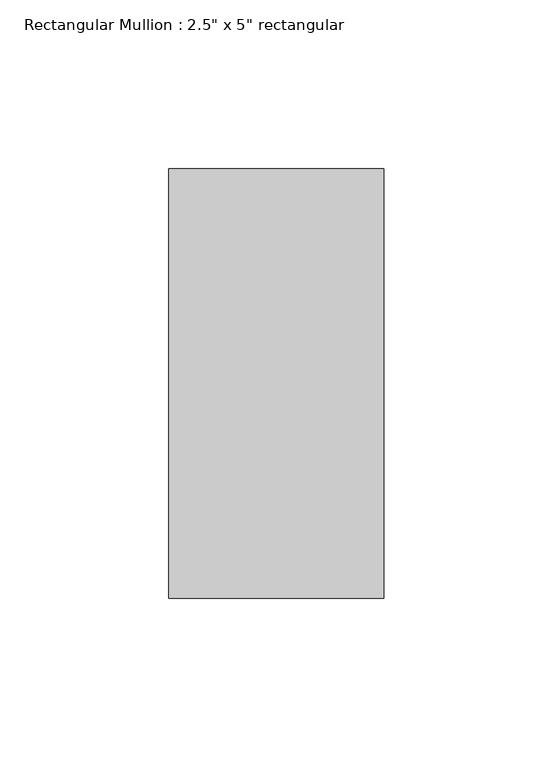
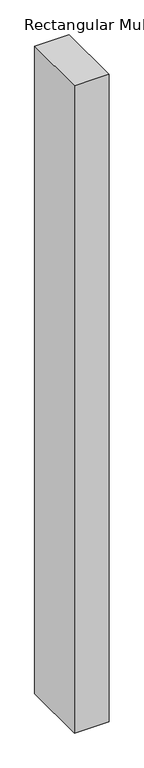
"""IFC4 building model written with IfcOpenShell, lengths in millimetres: member geometry."""

from ifc_helpers import new_model, si_unit, frame, origin, place, context, project, spatial, polyline, outline, extrude, source, transform, mapped, element, save


def member_05ffdb5f(model_context):
    return source(origin(), model_context, "Body", "SweptSolid", [
        extrude(outline(polyline([(0.0, 63.5), (0.0, -63.5), (-63.5, -63.5), (-63.5, 63.5), (0.0, 63.5)])), frame((0.0, 0.0, -1260.0620128), z_axis=(0.0, 0.0, 1.0), x_axis=(1.0, 0.0, 0.0)), (0.0, 0.0, 1.0), 1260.0620128),
    ])


if __name__ == "__main__":
    model = new_model("IFC4")
    model_context = context("Model", 3, world=origin())
    ifc_project = project(units=[si_unit("LENGTHUNIT", "METRE", prefix="MILLI")], contexts=[model_context])
    site = spatial("IfcSite", under=ifc_project)
    building = spatial("IfcBuilding", under=site)
    placement = place(None, origin())
    member_shape = member_05ffdb5f(model_context)
    element("IfcMember", 1, ObjectType="Rectangular Mullion : 2.5\" x 5\" rectangular", at=placement, inside=building, context=model_context, shape_type="MappedRepresentation", body=[
        mapped(member_shape, transform((0.0, 0.0, 0.0), x_axis=(1.0, 0.0, 0.0), y_axis=(0.0, 1.0, 0.0), z_axis=(0.0, 0.0, 1.0))),
    ])
    save(model, "model.ifc")

# Revit data of these elements
# Type "Rectangular Mullion : 2.5\" x 5\" rectangular"
#   built-in parameter 1007304 = 0.416667 (stored number, unit not read)
#   built-in parameter 1007301 = 0.104167 (stored number, unit not read)
#   built-in parameter 1007300 = 0.104167 (stored number, unit not read)
# Element 1 (IfcMember, "Rectangular Mullion : 2.5\" x 5\" rectangular")
#   Materials on its faces: "Aluminum"
# Materials
#   "Aluminum": class "Metal", colour RGB 247 247 247, transparency 0, Description = "Aluminum 6061", Cost = 0
